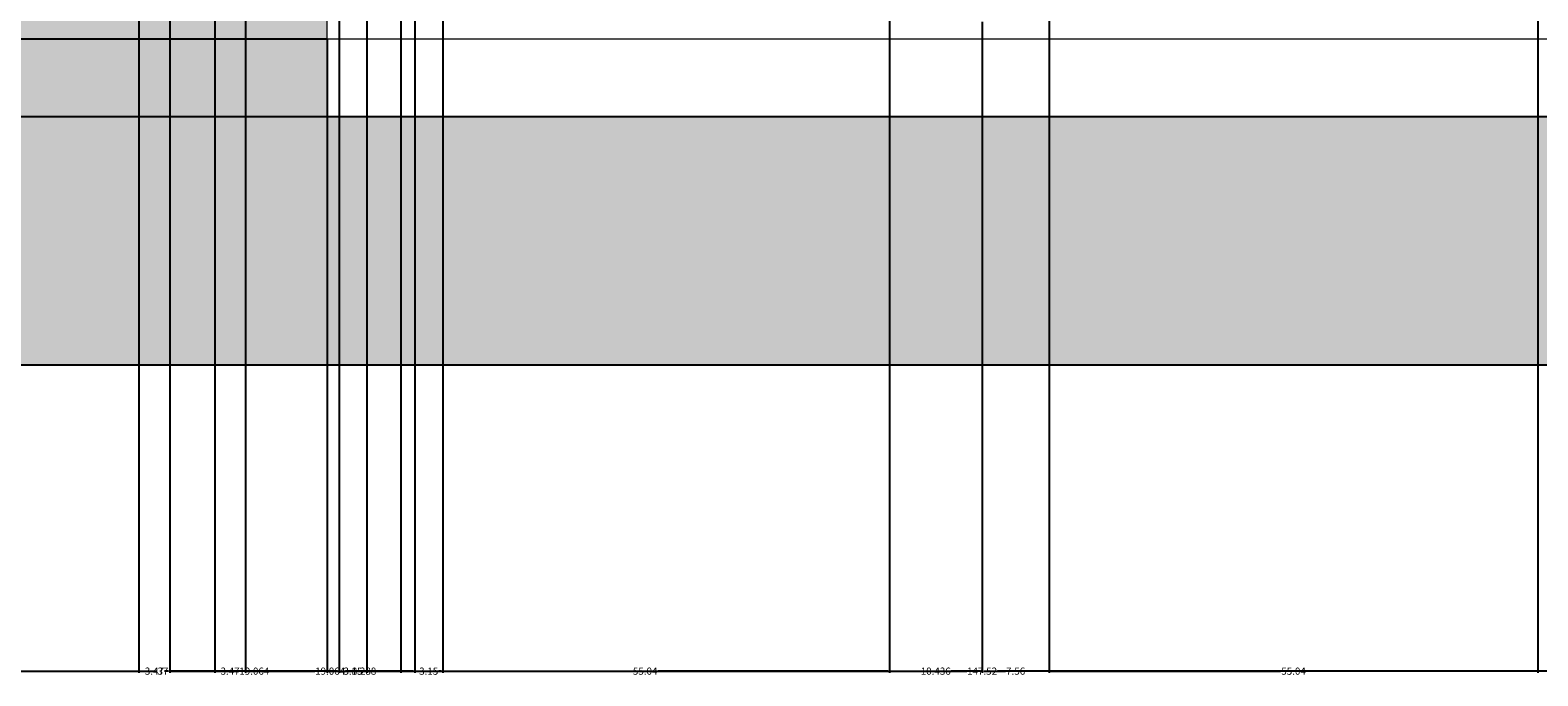
# Model space of a CAD drawing. Units: inches. Extents: x 36 to 594, y 79 to 831.
# Tile 4 of 30: x 221 to 390, y 79 to 152. Entities that reach past the tile are written whole.
import ezdxf

# ---------------------------------------------------------------- set-up
doc = ezdxf.new("R2010")
doc.units = ezdxf.units.IN
doc.header["$MEASUREMENT"] = 0
for name, color, linetype, lineweight in [('A-ANNO-DIMS', 2, 'Continuous', 18), ('A-DOOR', 3, 'Continuous', 18), ('A-ELEV', 7, 'Continuous', 25), ('A-ELEV-PATT', 8, 'Continuous', 13)]:
    doc.layers.add(name, color=color, linetype=linetype, lineweight=lineweight)
doc.styles.get("Standard").update_dxf_attribs({"font": 'arial.ttf'})
doc.dimstyles.get("Standard").update_dxf_attribs({"dimtxt": 0.8125, "dimasz": 0.18, "dimexe": 0.18, "dimexo": 0.0625, "dimgap": 0.09, "dimtad": 0, "dimtih": 1, "dimtoh": 1, "dimdec": 4, "dimzin": 0, "dimdsep": 46, "dimlunit": 4, "dimtxsty": 'Standard', "dimcen": 0.09, "dimadec": 0, "dimazin": 0, "dimtfac": 1, "dimtdec": 4, "dimtofl": 0, "dimtmove": 0, "dimatfit": 3, "dimfxl": 1, "dimtolj": 1, "dimtzin": 0, "dimarcsym": 0})

# ---------------------------------------------------------------- blocks, each defined once
blk = doc.blocks.new('*D9')
at = {"layer": 'A-ANNO-DIMS', "color": 0, "lineweight": -2, "transparency": 16777216}
for p, q in [((254.03, 142.15), (254.03, 79.53)), ((217.03, 114.15), (217.03, 79.53)), ((217.21, 79.71), (234.86, 79.71)), ((253.85, 79.71), (236.2, 79.71))]:
    blk.add_line(p, q, dxfattribs=at)
at = {"layer": 'A-ANNO-DIMS', "color": 0, "transparency": 16777216}
for points in [[(217.21, 79.74), (217.21, 79.68), (217.03, 79.71)], [(253.85, 79.74), (253.85, 79.68), (254.03, 79.71)]]:
    blk.add_solid(points, dxfattribs=at)
at = {"layer": 'Defpoints', "color": 0, "transparency": 16777216}
for p in [(254.03, 142.21), (217.03, 114.21), (254.03, 79.71)]:
    blk.add_point(p, dxfattribs=at)
at = {"layer": 'A-ANNO-DIMS', "color": 0, "transparency": 16777216, "insert": (235.53, 79.71), "char_height": 0.812, "attachment_point": 5}
blk.add_mtext('\\A1;37', dxfattribs=at)
blk = doc.blocks.new('*D10')
at = {"layer": 'A-ANNO-DIMS', "color": 0, "lineweight": -2, "transparency": 16777216}
for p, q in [((254.03, 142.15), (254.03, 79.53)), ((401.55, 142.15), (401.55, 79.53)), ((254.21, 79.71), (326.06, 79.71)), ((401.37, 79.71), (329.52, 79.71))]:
    blk.add_line(p, q, dxfattribs=at)
at = {"layer": 'A-ANNO-DIMS', "color": 0, "transparency": 16777216}
for points in [[(254.21, 79.74), (254.21, 79.68), (254.03, 79.71)], [(401.37, 79.74), (401.37, 79.68), (401.55, 79.71)]]:
    blk.add_solid(points, dxfattribs=at)
at = {"layer": 'Defpoints', "color": 0, "transparency": 16777216}
for p in [(254.03, 142.21), (401.55, 142.21), (401.55, 79.71)]:
    blk.add_point(p, dxfattribs=at)
at = {"layer": 'A-ANNO-DIMS', "color": 0, "transparency": 16777216, "insert": (327.79, 79.71), "char_height": 0.812, "attachment_point": 5}
blk.add_mtext('\\A1;147.52', dxfattribs=at)
blk = doc.blocks.new('*D28')
at = {"layer": 'A-ANNO-DIMS', "color": 0, "lineweight": -2, "transparency": 16777216}
for p, q in [((269.3, 796.05), (37.49, 796.05)), ((37.67, 795.87), (37.67, 455.63)), ((37.67, 114.39), (37.67, 454.62)), ((94.8, 114.21), (37.49, 114.21))]:
    blk.add_line(p, q, dxfattribs=at)
at = {"layer": 'A-ANNO-DIMS', "color": 0, "transparency": 16777216}
for points in [[(37.64, 795.87), (37.7, 795.87), (37.67, 796.05)], [(37.64, 114.39), (37.7, 114.39), (37.67, 114.21)]]:
    blk.add_solid(points, dxfattribs=at)
at = {"layer": 'Defpoints', "color": 0, "transparency": 16777216}
for p in [(37.67, 796.05), (269.36, 796.05), (94.87, 114.21)]:
    blk.add_point(p, dxfattribs=at)
at = {"layer": 'A-ANNO-DIMS', "color": 0, "transparency": 16777216, "insert": (37.67, 455.13), "char_height": 0.812, "attachment_point": 5}
blk.add_mtext('\\A1;681.8', dxfattribs=at)
blk = doc.blocks.new('*D78')
at = {"layer": 'A-ANNO-DIMS', "color": 0, "lineweight": -2, "transparency": 16777216}
for p, q in [((262.32, 162.93), (262.32, 79.53)), ((254.03, 150.87), (254.03, 79.53)), ((254.21, 79.71), (256.71, 79.71)), ((262.14, 79.71), (259.64, 79.71))]:
    blk.add_line(p, q, dxfattribs=at)
at = {"layer": 'A-ANNO-DIMS', "color": 0, "transparency": 16777216}
for points in [[(254.21, 79.74), (254.21, 79.68), (254.03, 79.71)], [(262.14, 79.74), (262.14, 79.68), (262.32, 79.71)]]:
    blk.add_solid(points, dxfattribs=at)
at = {"layer": 'Defpoints', "color": 0, "transparency": 16777216}
for p in [(262.32, 162.99), (254.03, 150.93), (262.32, 79.71)]:
    blk.add_point(p, dxfattribs=at)
at = {"layer": 'A-ANNO-DIMS', "color": 0, "transparency": 16777216, "insert": (258.17, 79.71), "char_height": 0.812, "attachment_point": 5}
blk.add_mtext('\\A1;8.288', dxfattribs=at)
blk = doc.blocks.new('*D79')
at = {"layer": 'A-ANNO-DIMS', "color": 0, "lineweight": -2, "transparency": 16777216}
for p, q in [((262.32, 162.93), (262.32, 79.53)), ((317.35, 162.93), (317.35, 79.53)), ((262.5, 79.71), (288.38, 79.71)), ((317.17, 79.71), (291.29, 79.71))]:
    blk.add_line(p, q, dxfattribs=at)
at = {"layer": 'A-ANNO-DIMS', "color": 0, "transparency": 16777216}
for points in [[(262.5, 79.74), (262.5, 79.68), (262.32, 79.71)], [(317.17, 79.74), (317.17, 79.68), (317.35, 79.71)]]:
    blk.add_solid(points, dxfattribs=at)
at = {"layer": 'Defpoints', "color": 0, "transparency": 16777216}
for p in [(262.32, 162.99), (317.35, 162.99), (317.35, 79.71)]:
    blk.add_point(p, dxfattribs=at)
at = {"layer": 'A-ANNO-DIMS', "color": 0, "transparency": 16777216, "insert": (289.84, 79.71), "char_height": 0.812, "attachment_point": 5}
blk.add_mtext('\\A1;55.04', dxfattribs=at)
blk = doc.blocks.new('*D80')
at = {"layer": 'A-ANNO-DIMS', "color": 0, "lineweight": -2, "transparency": 16777216}
for p, q in [((317.35, 162.93), (317.35, 79.53)), ((327.79, 152.87), (327.79, 79.53)), ((317.53, 79.71), (320.83, 79.71)), ((327.61, 79.71), (324.31, 79.71))]:
    blk.add_line(p, q, dxfattribs=at)
at = {"layer": 'A-ANNO-DIMS', "color": 0, "transparency": 16777216}
for points in [[(317.53, 79.74), (317.53, 79.68), (317.35, 79.71)], [(327.61, 79.74), (327.61, 79.68), (327.79, 79.71)]]:
    blk.add_solid(points, dxfattribs=at)
at = {"layer": 'Defpoints', "color": 0, "transparency": 16777216}
for p in [(317.35, 162.99), (327.79, 152.93), (327.79, 79.71)]:
    blk.add_point(p, dxfattribs=at)
at = {"layer": 'A-ANNO-DIMS', "color": 0, "transparency": 16777216, "insert": (322.57, 79.71), "char_height": 0.812, "attachment_point": 5}
blk.add_mtext('\\A1;10.436', dxfattribs=at)
blk = doc.blocks.new('*D81')
at = {"layer": 'A-ANNO-DIMS', "color": 0, "lineweight": -2, "transparency": 16777216}
for p, q in [((335.35, 162.93), (335.35, 79.53)), ((327.79, 152.87), (327.79, 79.53)), ((327.97, 79.71), (330.43, 79.71)), ((335.17, 79.71), (332.71, 79.71))]:
    blk.add_line(p, q, dxfattribs=at)
at = {"layer": 'A-ANNO-DIMS', "color": 0, "transparency": 16777216}
for points in [[(327.97, 79.74), (327.97, 79.68), (327.79, 79.71)], [(335.17, 79.74), (335.17, 79.68), (335.35, 79.71)]]:
    blk.add_solid(points, dxfattribs=at)
at = {"layer": 'Defpoints', "color": 0, "transparency": 16777216}
for p in [(335.35, 162.99), (327.79, 152.93), (335.35, 79.71)]:
    blk.add_point(p, dxfattribs=at)
at = {"layer": 'A-ANNO-DIMS', "color": 0, "transparency": 16777216, "insert": (331.57, 79.71), "char_height": 0.812, "attachment_point": 5}
blk.add_mtext('\\A1;7.56', dxfattribs=at)
blk = doc.blocks.new('*D82')
at = {"layer": 'A-ANNO-DIMS', "color": 0, "lineweight": -2, "transparency": 16777216}
for p, q in [((335.35, 162.93), (335.35, 79.53)), ((390.39, 162.93), (390.39, 79.53)), ((335.53, 79.71), (361.41, 79.71)), ((390.21, 79.71), (364.33, 79.71))]:
    blk.add_line(p, q, dxfattribs=at)
at = {"layer": 'A-ANNO-DIMS', "color": 0, "transparency": 16777216}
for points in [[(335.53, 79.74), (335.53, 79.68), (335.35, 79.71)], [(390.21, 79.74), (390.21, 79.68), (390.39, 79.71)]]:
    blk.add_solid(points, dxfattribs=at)
at = {"layer": 'Defpoints', "color": 0, "transparency": 16777216}
for p in [(335.35, 162.99), (390.39, 162.99), (390.39, 79.71)]:
    blk.add_point(p, dxfattribs=at)
at = {"layer": 'A-ANNO-DIMS', "color": 0, "transparency": 16777216, "insert": (362.87, 79.71), "char_height": 0.812, "attachment_point": 5}
blk.add_mtext('\\A1;55.04', dxfattribs=at)
blk = doc.blocks.new('*D90')
at = {"layer": 'A-ANNO-DIMS', "color": 0, "lineweight": -2, "transparency": 16777216}
for p, q in [((255.97, 269.61), (37.49, 269.61)), ((37.67, 269.43), (37.67, 210.78)), ((37.67, 151.11), (37.67, 209.77)), ((253.97, 150.93), (37.49, 150.93))]:
    blk.add_line(p, q, dxfattribs=at)
at = {"layer": 'A-ANNO-DIMS', "color": 0, "transparency": 16777216}
for points in [[(37.64, 269.43), (37.7, 269.43), (37.67, 269.61)], [(37.64, 151.11), (37.7, 151.11), (37.67, 150.93)]]:
    blk.add_solid(points, dxfattribs=at)
at = {"layer": 'Defpoints', "color": 0, "transparency": 16777216}
for p in [(37.67, 269.61), (256.03, 269.61), (254.03, 150.93)]:
    blk.add_point(p, dxfattribs=at)
at = {"layer": 'A-ANNO-DIMS', "color": 0, "transparency": 16777216, "insert": (37.67, 210.27), "char_height": 0.812, "attachment_point": 5}
blk.add_mtext('\\A1;118.67', dxfattribs=at)
blk = doc.blocks.new('*D96')
at = {"layer": 'A-ANNO-DIMS', "color": 0, "lineweight": -2, "transparency": 16777216}
for p, q in [((236.29, 484.36), (236.29, 79.53)), ((232.82, 475.35), (232.82, 79.53)), ((233, 79.71), (233.41, 79.71)), ((236.11, 79.71), (235.7, 79.71))]:
    blk.add_line(p, q, dxfattribs=at)
at = {"layer": 'A-ANNO-DIMS', "color": 0, "transparency": 16777216}
for points in [[(233, 79.74), (233, 79.68), (232.82, 79.71)], [(236.11, 79.74), (236.11, 79.68), (236.29, 79.71)]]:
    blk.add_solid(points, dxfattribs=at)
at = {"layer": 'Defpoints', "color": 0, "transparency": 16777216}
for p in [(236.29, 484.42), (232.82, 475.41), (236.29, 79.71)]:
    blk.add_point(p, dxfattribs=at)
at = {"layer": 'A-ANNO-DIMS', "color": 0, "transparency": 16777216, "insert": (234.56, 79.71), "char_height": 0.812, "attachment_point": 5}
blk.add_mtext('\\A1;3.47', dxfattribs=at)
blk = doc.blocks.new('*D97')
at = {"layer": 'A-ANNO-DIMS', "color": 0, "lineweight": -2, "transparency": 16777216}
for p, q in [((236.29, 484.36), (236.29, 79.53)), ((255.36, 484.36), (255.36, 79.53)), ((236.47, 79.71), (244.09, 79.71)), ((255.18, 79.71), (247.56, 79.71))]:
    blk.add_line(p, q, dxfattribs=at)
at = {"layer": 'A-ANNO-DIMS', "color": 0, "transparency": 16777216}
for points in [[(236.47, 79.74), (236.47, 79.68), (236.29, 79.71)], [(255.18, 79.74), (255.18, 79.68), (255.36, 79.71)]]:
    blk.add_solid(points, dxfattribs=at)
at = {"layer": 'Defpoints', "color": 0, "transparency": 16777216}
for p in [(236.29, 484.42), (255.36, 484.42), (255.36, 79.71)]:
    blk.add_point(p, dxfattribs=at)
at = {"layer": 'A-ANNO-DIMS', "color": 0, "transparency": 16777216, "insert": (245.82, 79.71), "char_height": 0.812, "attachment_point": 5}
blk.add_mtext('\\A1;19.064', dxfattribs=at)
blk = doc.blocks.new('*D98')
at = {"layer": 'A-ANNO-DIMS', "color": 0, "lineweight": -2, "transparency": 16777216}
for p, q in [((255.36, 484.36), (255.36, 79.53)), ((258.51, 475.35), (258.51, 79.53)), ((255.54, 79.71), (255.78, 79.71)), ((258.33, 79.71), (258.08, 79.71))]:
    blk.add_line(p, q, dxfattribs=at)
at = {"layer": 'A-ANNO-DIMS', "color": 0, "transparency": 16777216}
for points in [[(255.54, 79.74), (255.54, 79.68), (255.36, 79.71)], [(258.33, 79.74), (258.33, 79.68), (258.51, 79.71)]]:
    blk.add_solid(points, dxfattribs=at)
at = {"layer": 'Defpoints', "color": 0, "transparency": 16777216}
for p in [(255.36, 484.42), (258.51, 475.41), (258.51, 79.71)]:
    blk.add_point(p, dxfattribs=at)
at = {"layer": 'A-ANNO-DIMS', "color": 0, "transparency": 16777216, "insert": (256.93, 79.71), "char_height": 0.812, "attachment_point": 5}
blk.add_mtext('\\A1;3.15', dxfattribs=at)
blk = doc.blocks.new('*D108')
at = {"layer": 'A-ANNO-DIMS', "color": 0, "lineweight": -2, "transparency": 16777216}
for p, q in [((244.82, 364.03), (244.82, 79.53)), ((241.36, 355.02), (241.36, 79.53)), ((241.54, 79.71), (241.95, 79.71)), ((244.64, 79.71), (244.24, 79.71))]:
    blk.add_line(p, q, dxfattribs=at)
at = {"layer": 'A-ANNO-DIMS', "color": 0, "transparency": 16777216}
for points in [[(241.54, 79.74), (241.54, 79.68), (241.36, 79.71)], [(244.64, 79.74), (244.64, 79.68), (244.82, 79.71)]]:
    blk.add_solid(points, dxfattribs=at)
at = {"layer": 'Defpoints', "color": 0, "transparency": 16777216}
for p in [(244.82, 364.09), (241.36, 355.08), (244.82, 79.71)]:
    blk.add_point(p, dxfattribs=at)
at = {"layer": 'A-ANNO-DIMS', "color": 0, "transparency": 16777216, "insert": (243.09, 79.71), "char_height": 0.812, "attachment_point": 5}
blk.add_mtext('\\A1;3.47', dxfattribs=at)
blk = doc.blocks.new('*D109')
at = {"layer": 'A-ANNO-DIMS', "color": 0, "lineweight": -2, "transparency": 16777216}
for p, q in [((244.82, 364.03), (244.82, 79.53)), ((263.89, 364.03), (263.89, 79.53)), ((245, 79.71), (252.62, 79.71)), ((263.71, 79.71), (256.09, 79.71))]:
    blk.add_line(p, q, dxfattribs=at)
at = {"layer": 'A-ANNO-DIMS', "color": 0, "transparency": 16777216}
for points in [[(245, 79.74), (245, 79.68), (244.82, 79.71)], [(263.71, 79.74), (263.71, 79.68), (263.89, 79.71)]]:
    blk.add_solid(points, dxfattribs=at)
at = {"layer": 'Defpoints', "color": 0, "transparency": 16777216}
for p in [(244.82, 364.09), (263.89, 364.09), (263.89, 79.71)]:
    blk.add_point(p, dxfattribs=at)
at = {"layer": 'A-ANNO-DIMS', "color": 0, "transparency": 16777216, "insert": (254.36, 79.71), "char_height": 0.812, "attachment_point": 5}
blk.add_mtext('\\A1;19.064', dxfattribs=at)
blk = doc.blocks.new('*D110')
at = {"layer": 'A-ANNO-DIMS', "color": 0, "lineweight": -2, "transparency": 16777216}
for p, q in [((263.89, 364.03), (263.89, 79.53)), ((267.04, 355.02), (267.04, 79.53)), ((264.07, 79.71), (264.32, 79.71)), ((266.86, 79.71), (266.61, 79.71))]:
    blk.add_line(p, q, dxfattribs=at)
at = {"layer": 'A-ANNO-DIMS', "color": 0, "transparency": 16777216}
for points in [[(264.07, 79.74), (264.07, 79.68), (263.89, 79.71)], [(266.86, 79.74), (266.86, 79.68), (267.04, 79.71)]]:
    blk.add_solid(points, dxfattribs=at)
at = {"layer": 'Defpoints', "color": 0, "transparency": 16777216}
for p in [(263.89, 364.09), (267.04, 355.08), (267.04, 79.71)]:
    blk.add_point(p, dxfattribs=at)
at = {"layer": 'A-ANNO-DIMS', "color": 0, "transparency": 16777216, "insert": (265.46, 79.71), "char_height": 0.812, "attachment_point": 5}
blk.add_mtext('\\A1;3.15', dxfattribs=at)

msp = doc.modelspace()

# ---------------------------------------------------------------- hatches: boundary and pattern name
at = {"layer": 'A-ELEV-PATT'}
h = msp.add_hatch(color=256, dxfattribs=at)
h.dxf.hatch_style = 1
h.paths.add_polyline_path([(398.0873, 796.0465), (269.3592, 796.0465), (269.3592, 770.1455), (397.8159, 770.1455)])
h.paths.add_polyline_path([(397.7518, 764.0341), (269.3592, 764.0341), (269.3592, 630.0394), (341.8367, 630.0394), (341.8367, 720.595), (335.0881, 728.3699), (329.982, 735.3373), (345.3661, 727.7743), (397.1052, 702.3389)])
h.paths.add_polyline_path([(341.8367, 594.2124), (201.4189, 594.2124), (201.4189, 475.4136), (232.8216, 475.4136), (232.8216, 524.6037), (341.8367, 524.6037)])
h.paths.add_polyline_path([(177.525, 594.2124), (118.7598, 594.2124), (118.7598, 450.2124), (177.525, 450.2124)])
h.paths.add_polyline_path([(424.4958, 594.2124), (365.7306, 594.2124), (365.7306, 450.2124), (424.4958, 450.2124)])
h.paths.add_polyline_path([(241.3553, 404.2737), (355.8569, 404.2737), (355.8569, 355.0836), (424.5492, 355.0836), (424.5492, 425.7333), (118.7598, 426.2844), (118.7598, 355.0836), (241.3553, 355.0836)])
h.paths.add_polyline_path([(448.3898, 306.2124), (217.0273, 306.2124), (217.0273, 142.2124), (254.0293, 142.2124), (254.0293, 150.9347), (254.0293, 286.1802), (401.5491, 286.1802), (401.5491, 150.9347), (401.5491, 142.2124), (448.3898, 142.2124)])
h.paths.add_polyline_path([(448.3898, 142.2124), (401.5491, 142.2124), (217.0273, 142.2124), (217.0273, 114.2124), (448.3898, 114.2124)])
h.paths.add_polyline_path([(217.0273, 306.2124), (174.7353, 306.2124), (94.8658, 306.2124), (94.8658, 162.2124), (103.3368, 162.2124), (103.3368, 264.6224), (103.3368, 286.1802), (217.0273, 286.1802)])

# ---------------------------------------------------------------- linework, layer by layer
at = {"layer": 'A-DOOR'}
msp.add_lwpolyline([(254.0293, 286.1802), (401.5491, 286.1802), (401.5491, 150.9347), (254.0293, 150.9347)], close=True, dxfattribs=at)
at = {"layer": 'A-ELEV'}
for p, q in [((254.0293, 150.9347), (254.0293, 142.2124)), ((174.7353, 142.2124), (448.3898, 142.2124)), ((84.3711, 114.2124), (558.1689, 114.2124))]:
    msp.add_line(p, q, dxfattribs=at)

# ---------------------------------------------------------------- dimensions: what is measured, and where the dimension line sits
at = {"layer": 'A-ANNO-DIMS'}
for base, p1, p2, override, picture, middle in [((37.6733, 796.0465), (94.8658, 114.2124), (269.3592, 796.0465), {"dimdec": 1, "dimlfac": 1, "dimrnd": 0, "dimzin": 0, "dimdsep": 46, "dimlunit": 2}, '*D28', (37.6733, 455.1294)), ((37.6733, 269.6084), (254.0293, 150.9347), (256.0293, 269.6084), {"dimdec": 2, "dimlfac": 1, "dimrnd": 0, "dimzin": 0, "dimdsep": 46, "dimlunit": 2}, '*D90', (37.6733, 210.2716))]:
    dim = msp.add_linear_dim(base=base, p1=p1, p2=p2, angle=90, dimstyle='Standard', override=override, dxfattribs=at)
    dim.commit()
    dim.dimension.update_dxf_attribs({"geometry": picture, "text_midpoint": middle})
for base, p1, p2, override, picture, middle in [((236.2911, 79.7124), (232.8216, 475.4136), (236.2911, 484.4187), {"dimdec": 2, "dimlfac": 1, "dimrnd": 0, "dimzin": 0, "dimdsep": 46, "dimlunit": 2}, '*D96', (234.5563, 79.7124)), ((255.3555, 79.7124), (236.2911, 484.4187), (255.3555, 484.4187), {"dimdec": 3, "dimlfac": 1, "dimrnd": 0, "dimzin": 0, "dimdsep": 46, "dimlunit": 2}, '*D97', (245.8233, 79.7124)), ((258.5056, 79.7124), (255.3555, 484.4187), (258.5056, 475.4136), {"dimdec": 2, "dimlfac": 1, "dimrnd": 0, "dimzin": 0, "dimdsep": 46, "dimlunit": 2}, '*D98', (256.9305, 79.7124)), ((244.8248, 79.7124), (241.3553, 355.0836), (244.8248, 364.0887), {"dimdec": 2, "dimlfac": 1, "dimrnd": 0, "dimzin": 0, "dimdsep": 46, "dimlunit": 2}, '*D108', (243.09, 79.7124)), ((263.8892, 79.7124), (244.8248, 364.0887), (263.8892, 364.0887), {"dimdec": 3, "dimlfac": 1, "dimrnd": 0, "dimzin": 0, "dimdsep": 46, "dimlunit": 2}, '*D109', (254.357, 79.7124)), ((267.0393, 79.7124), (263.8892, 364.0887), (267.0393, 355.0836), {"dimdec": 2, "dimlfac": 1, "dimrnd": 0, "dimzin": 0, "dimdsep": 46, "dimlunit": 2}, '*D110', (265.4643, 79.7124)), ((262.3169, 79.7124), (254.0293, 150.9347), (262.3169, 162.9881), {"dimdec": 3, "dimlfac": 1, "dimrnd": 0, "dimzin": 0, "dimdsep": 46, "dimlunit": 2}, '*D78', (258.1731, 79.7124)), ((317.3533, 79.7124), (262.3169, 162.9881), (317.3533, 162.9881), {"dimdec": 2, "dimlfac": 1, "dimrnd": 0, "dimzin": 0, "dimdsep": 46, "dimlunit": 2}, '*D79', (289.8351, 79.7124)), ((327.7892, 79.7124), (317.3533, 162.9881), (327.7892, 152.9347), {"dimdec": 3, "dimlfac": 1, "dimrnd": 0, "dimzin": 0, "dimdsep": 46, "dimlunit": 2}, '*D80', (322.5712, 79.7124)), ((335.3496, 79.7124), (327.7892, 152.9347), (335.3496, 162.9881), {"dimdec": 2, "dimlfac": 1, "dimrnd": 0, "dimzin": 0, "dimdsep": 46, "dimlunit": 2}, '*D81', (331.5694, 79.7124)), ((390.386, 79.7124), (335.3496, 162.9881), (390.386, 162.9881), {"dimdec": 2, "dimlfac": 1, "dimrnd": 0, "dimzin": 0, "dimdsep": 46, "dimlunit": 2}, '*D82', (362.8678, 79.7124)), ((254.0293, 79.7124), (217.0273, 114.2124), (254.0293, 142.2124), {"dimdec": 0, "dimlfac": 1, "dimrnd": 0, "dimzin": 0, "dimdsep": 46, "dimlunit": 2}, '*D9', (235.5283, 79.7124)), ((401.5491, 79.7124), (254.0293, 142.2124), (401.5491, 142.2124), {"dimdec": 2, "dimlfac": 1, "dimrnd": 0, "dimzin": 0, "dimdsep": 46, "dimlunit": 2}, '*D10', (327.7892, 79.7124))]:
    dim = msp.add_linear_dim(base=base, p1=p1, p2=p2, dimstyle='Standard', override=override, dxfattribs=at)
    dim.commit()
    dim.dimension.update_dxf_attribs({"geometry": picture, "text_midpoint": middle})

doc.saveas('drawing.dxf')
